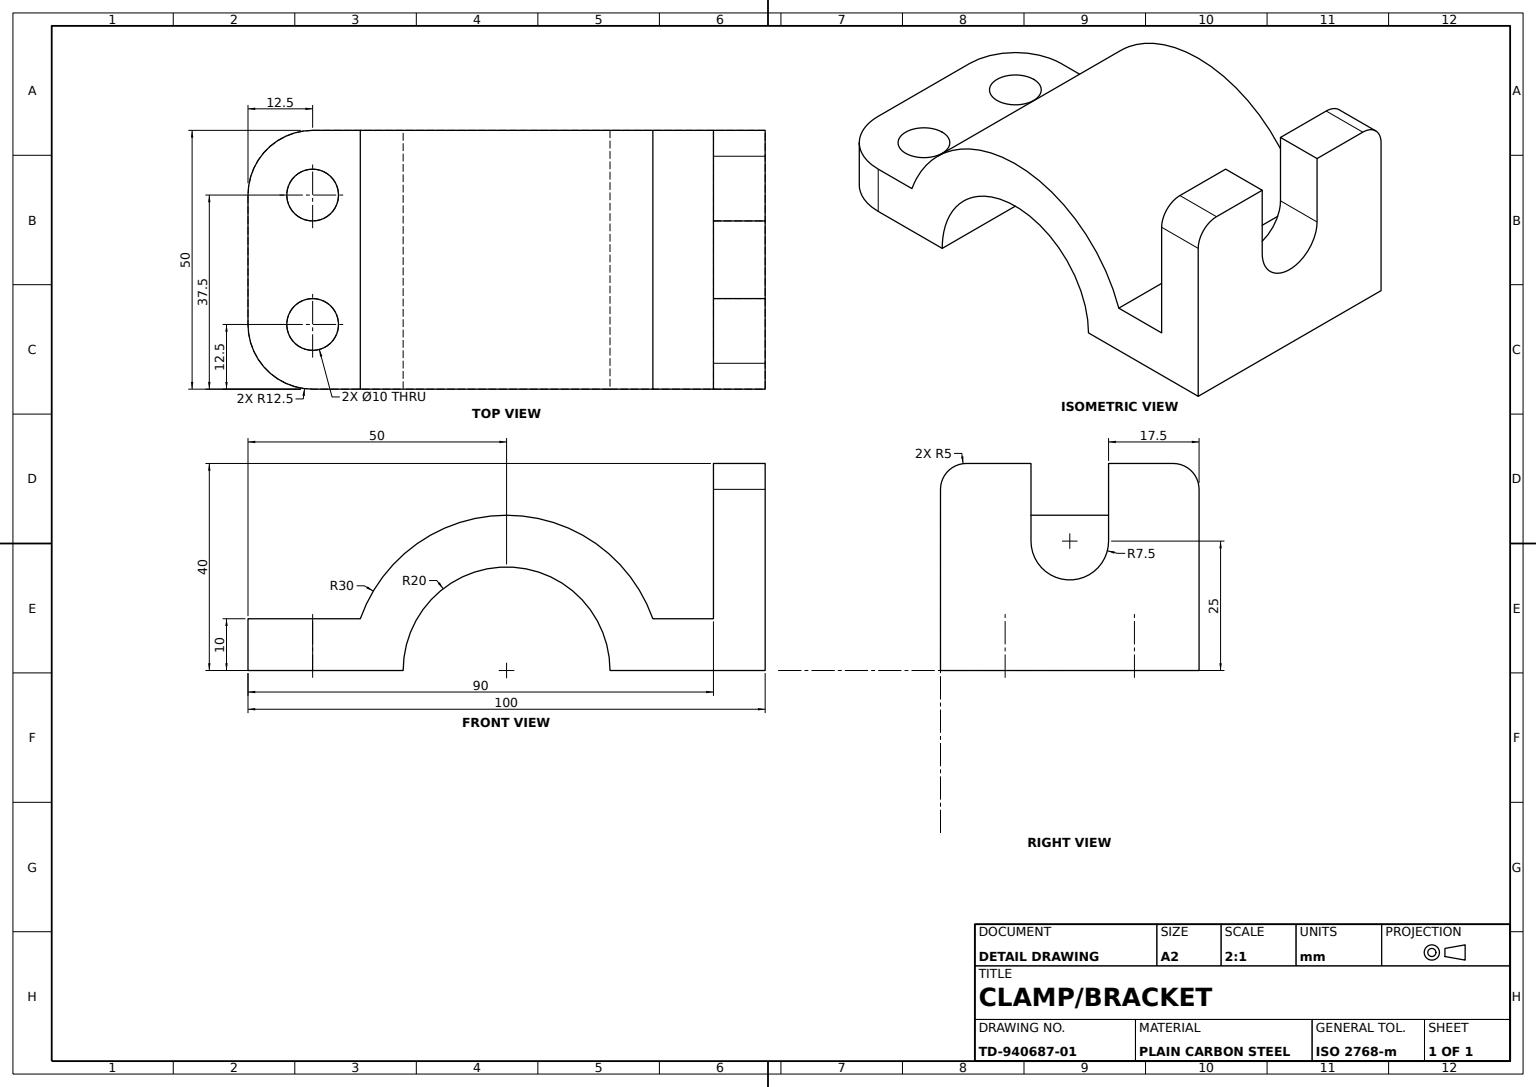
from build123d import *

# Parameters (mm, degrees)
ARCH_BODY_DEPTH             = 50
SIDE_RELIEF_CUT_DEPTH       = 50
END_RELIEF_CUT_DEPTH        = 50
ARCH_BORE_CUT_DEPTH         = 50
LUG_BLOCK_DEPTH             = 50
LUG_U_SLOT_DEPTH            = 50
FLANGE_BOLT_HOLES_PROFILE_R = 5
FLANGE_BOLT_HOLES_DEPTH     = 50


with BuildPart() as part:
    # Arch Body Profile → Arch Body (new body)
    with BuildSketch(Plane.XY):
        Polygon((0, 0), (100, 0), (100, 40), (90, 40), (90, 10), (0, 10), align=None)
    extrude(amount=ARCH_BODY_DEPTH)

    # Side Relief Profile → Side Relief Cut (cut)
    with BuildSketch(Plane(origin=(100, 0, 0), x_dir=(0, 0, -1), z_dir=(1, 0, 0))):
        with BuildLine():
            Line((-50, 40), (-50, 35))
            ThreePointArc((-50, 35), (-48.535533906, 38.535533906), (-45, 40))
            Line((-45, 40), (-50, 40))
        make_face()
        with BuildLine():
            Line((0, 40), (0, 35))
            ThreePointArc((0, 35), (-1.464466094, 38.535533906), (-5, 40))
            Line((-5, 40), (0, 40))
        make_face()
    extrude(amount=-SIDE_RELIEF_CUT_DEPTH, mode=Mode.SUBTRACT)

    # End Relief Profile → End Relief Cut (cut)
    with BuildSketch(Plane(origin=(100, 0, 0), x_dir=(0, 0, -1), z_dir=(1, 0, 0))):
        with BuildLine():
            Line((-17.5, 40), (-25, 40))
            Line((-25, 40), (-32.5, 40))
            Line((-32.5, 40), (-32.5, 25))
            ThreePointArc((-32.5, 25), (-25, 17.5), (-17.5, 25))
            Line((-17.5, 25), (-17.5, 40))
        make_face()
    extrude(amount=-END_RELIEF_CUT_DEPTH, mode=Mode.SUBTRACT)

    # Arch Bore Profile → Arch Bore Cut (cut)
    with BuildSketch(Plane(origin=(0, 10, 0), x_dir=(1, 0, 0), z_dir=(0, 1, 0))):
        with BuildLine():
            Line((0, -50), (12.5, -50))
            ThreePointArc((12.5, -50), (3.661165235, -46.338834765), (0, -37.5))
            Line((0, -37.5), (0, -50))
        make_face()
        with BuildLine():
            Line((0, 0), (12.5, 0))
            ThreePointArc((12.5, 0), (3.661165235, -3.661165235), (0, -12.5))
            Line((0, -12.5), (0, 0))
        make_face()
    extrude(amount=-ARCH_BORE_CUT_DEPTH, mode=Mode.SUBTRACT)

    # Lug Block Profile → Lug Block (add)
    with BuildSketch(Plane.XY.offset(50)):
        with BuildLine():
            Line((21.715728753, 10), (78.284271247, 10))
            ThreePointArc((78.284271247, 10), (50, 30), (21.715728753, 10))
        make_face()
    extrude(amount=-LUG_BLOCK_DEPTH)

    # Lug U-Slot Profile → Lug U-Slot (cut)
    with BuildSketch(Plane.XY.offset(50)):
        with BuildLine():
            Line((30, 0), (70, 0))
            ThreePointArc((70, 0), (50, 20), (30, 0))
        make_face()
    extrude(amount=-LUG_U_SLOT_DEPTH, mode=Mode.SUBTRACT)

    # Flange Bolt Holes Profile → Flange Bolt Holes (cut)
    with BuildSketch(Plane(origin=(0, 10, 0), x_dir=(1, 0, 0), z_dir=(0, 1, 0))):
        with Locations(Location((12.5, -37.5, 0), (0, 0, 270))):
            Circle(FLANGE_BOLT_HOLES_PROFILE_R)
        with Locations(Location((12.5, -12.5, 0), (0, 0, 270))):
            Circle(FLANGE_BOLT_HOLES_PROFILE_R)
    extrude(amount=-FLANGE_BOLT_HOLES_DEPTH, mode=Mode.SUBTRACT)


solid = part.part
